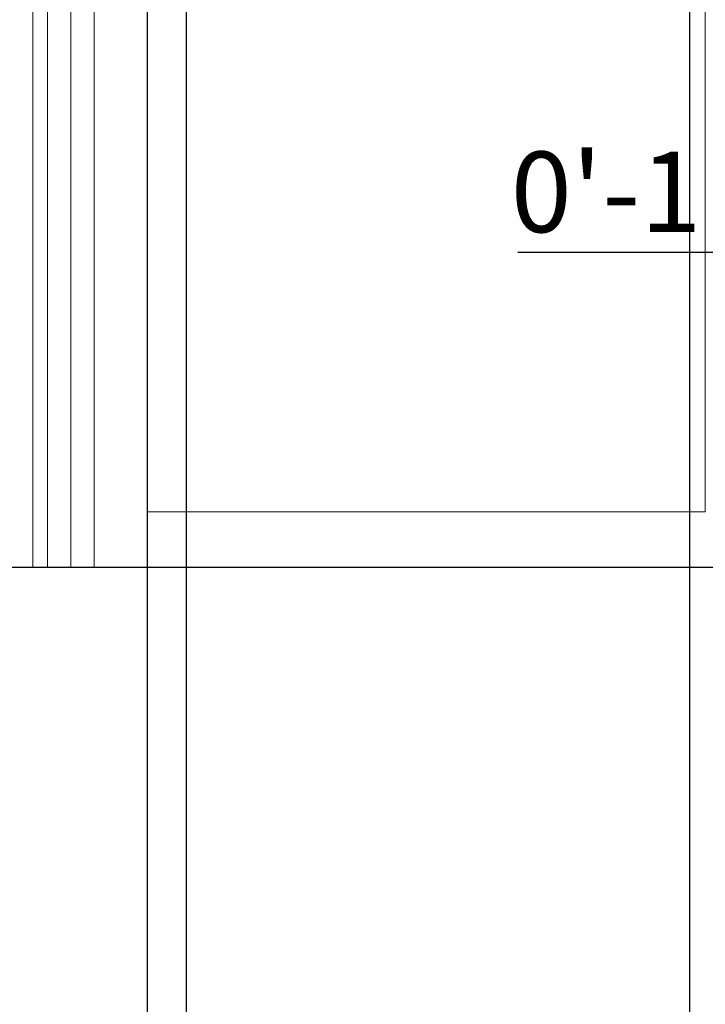
# Model space of a CAD drawing. Units: inches. Extents: x 2656 to 9931, y 1941 to 3068.
# Tile 30 of 46: x 2817 to 2868, y 2855 to 2929. Entities that reach past the tile are written whole.
import ezdxf

# ---------------------------------------------------------------- set-up
doc = ezdxf.new("R2010")
doc.units = ezdxf.units.IN
for name, color, linetype, lineweight in [('A-ANNO-DIMS', 2, 'Continuous', 18), ('A-ELEV', 7, 'Continuous', 25), ('A-ELEV-FNSH', 8, 'Continuous', 13)]:
    doc.layers.add(name, color=color, linetype=linetype, lineweight=lineweight)
doc.styles.get("Standard").update_dxf_attribs({"font": 'arial.ttf'})
doc.dimstyles.new('ISO-25', dxfattribs={"dimtxt": 6, "dimasz": 2.5, "dimexe": 1.25, "dimexo": 0.625, "dimtad": 1, "dimdec": 0, "dimlunit": 3, "dimtxsty": 'Standard', "dimcen": 2.5, "dimadec": 0, "dimazin": 0, "dimtfac": 1, "dimtdec": 0, "dimtmove": 0, "dimatfit": 3, "dimfxl": 1, "dimarcsym": 0})

# ---------------------------------------------------------------- blocks, each defined once
blk = doc.blocks.new('*D63')
at = {"layer": 'A-ANNO-DIMS', "color": 0, "lineweight": -2, "transparency": 16777216}
for p, q in [((2807.088, 2803.318), (2807.088, 2893.004)), ((2799.699, 2803.318), (2808.338, 2803.318)), ((2807.088, 2752.393), (2807.088, 2800.818)), ((2799.699, 2749.893), (2808.338, 2749.893))]:
    blk.add_line(p, q, dxfattribs=at)
at = {"layer": 'A-ANNO-DIMS', "color": 0, "transparency": 16777216}
for points in [[(2806.671, 2800.818), (2807.505, 2800.818), (2807.088, 2803.318)], [(2806.671, 2752.393), (2807.505, 2752.393), (2807.088, 2749.893)]]:
    blk.add_solid(points, dxfattribs=at)
at = {"layer": 'Defpoints', "color": 0, "transparency": 16777216}
for p in [(2799.074, 2803.318), (2807.088, 2803.318), (2799.074, 2749.893)]:
    blk.add_point(p, dxfattribs=at)
at = {"layer": 'A-ANNO-DIMS', "color": 0, "transparency": 16777216, "insert": (2803.358, 2849.411), "char_height": 6, "attachment_point": 5, "rotation": 90}
blk.add_mtext('FRONT GATE 4\'-5 1/2"', dxfattribs=at)
blk = doc.blocks.new('*D151')
at = {"layer": 'A-ANNO-DIMS', "color": 0, "lineweight": -2, "transparency": 16777216}
for p, q in [((2829.546, 2956.424), (2829.546, 2703.709)), ((2867.059, 2955.98), (2867.059, 2703.709)), ((2832.046, 2704.959), (2864.559, 2704.959))]:
    blk.add_line(p, q, dxfattribs=at)
at = {"layer": 'A-ANNO-DIMS', "color": 0, "transparency": 16777216}
for points in [[(2832.046, 2705.376), (2832.046, 2704.543), (2829.546, 2704.959)], [(2864.559, 2705.376), (2864.559, 2704.543), (2867.059, 2704.959)]]:
    blk.add_solid(points, dxfattribs=at)
at = {"layer": 'Defpoints', "color": 0, "transparency": 16777216}
for p in [(2829.546, 2957.049), (2867.059, 2956.605), (2867.059, 2704.959)]:
    blk.add_point(p, dxfattribs=at)
at = {"layer": 'A-ANNO-DIMS', "color": 0, "transparency": 16777216, "insert": (2848.302, 2708.689), "char_height": 6, "attachment_point": 5}
blk.add_mtext('3\'-1 1/2"', dxfattribs=at)
blk = doc.blocks.new('*D153')
at = {"layer": 'A-ANNO-DIMS', "color": 0, "lineweight": -2, "transparency": 16777216}
for p, q in [((2826.64, 2993.722), (2826.64, 2703.709)), ((2829.546, 2956.424), (2829.546, 2703.709)), ((2824.14, 2704.959), (2821.64, 2704.959)), ((2826.64, 2704.959), (2829.546, 2704.959)), ((2832.046, 2704.959), (2851.745, 2704.959))]:
    blk.add_line(p, q, dxfattribs=at)
at = {"layer": 'A-ANNO-DIMS', "color": 0, "transparency": 16777216}
for points in [[(2824.14, 2705.376), (2824.14, 2704.543), (2826.64, 2704.959)], [(2832.046, 2705.376), (2832.046, 2704.543), (2829.546, 2704.959)]]:
    blk.add_solid(points, dxfattribs=at)
at = {"layer": 'Defpoints', "color": 0, "transparency": 16777216}
for p in [(2826.64, 2994.347), (2829.546, 2957.049), (2829.546, 2704.959)]:
    blk.add_point(p, dxfattribs=at)
at = {"layer": 'A-ANNO-DIMS', "color": 0, "transparency": 16777216, "insert": (2843.145, 2708.65), "char_height": 6, "attachment_point": 5}
blk.add_mtext('0\'-3"', dxfattribs=at)
blk = doc.blocks.new('*D163')
at = {"layer": 'A-ANNO-DIMS', "color": 0, "lineweight": -2, "transparency": 16777216}
for p, q in [((2890.428, 2926.692), (2890.428, 2910.117)), ((2891.822, 2926.692), (2891.822, 2910.117)), ((2887.928, 2911.367), (2854.248, 2911.367)), ((2891.822, 2911.367), (2890.428, 2911.367)), ((2894.322, 2911.367), (2896.822, 2911.367))]:
    blk.add_line(p, q, dxfattribs=at)
at = {"layer": 'A-ANNO-DIMS', "color": 0, "transparency": 16777216}
for points in [[(2887.928, 2911.784), (2887.928, 2910.951), (2890.428, 2911.367)], [(2894.322, 2911.784), (2894.322, 2910.951), (2891.822, 2911.367)]]:
    blk.add_solid(points, dxfattribs=at)
at = {"layer": 'Defpoints', "color": 0, "transparency": 16777216}
for p in [(2890.428, 2927.317), (2891.822, 2927.317), (2890.428, 2911.367)]:
    blk.add_point(p, dxfattribs=at)
at = {"layer": 'A-ANNO-DIMS', "color": 0, "transparency": 16777216, "insert": (2869.838, 2915.095), "char_height": 6, "attachment_point": 5}
blk.add_mtext('0\'-1 1/2"', dxfattribs=at)

msp = doc.modelspace()

# ---------------------------------------------------------------- linework, layer by layer
at = {"layer": 'A-ELEV'}
msp.add_line((2998.157, 2887.893), (2743.157, 2887.893), dxfattribs=at)
at = {"layer": 'A-ELEV-FNSH'}
for p, q in [((2818.129, 2887.893), (2818.129, 2998.286)), ((2819.227, 2887.893), (2819.227, 2998.286)), ((2820.954, 2887.893), (2820.954, 2998.286)), ((2822.705, 2887.893), (2822.705, 2998.286))]:
    msp.add_line(p, q, dxfattribs=at)
msp.add_lwpolyline([(2826.64, 2994.347), (2868.226, 2994.347), (2868.226, 2892.035), (2826.64, 2892.035)], close=True, dxfattribs=at)

# ---------------------------------------------------------------- dimensions: what is measured, and where the dimension line sits
at = {"layer": 'A-ANNO-DIMS'}
for base, p1, p2, picture, middle in [((2829.546, 2704.959), (2826.64, 2994.347), (2829.546, 2957.049), '*D153', (2843.145, 2708.65)), ((2867.059, 2704.959), (2829.546, 2957.049), (2867.059, 2956.605), '*D151', (2848.302, 2708.689))]:
    dim = msp.add_linear_dim(base=base, p1=p1, p2=p2, dimstyle='ISO-25', override={"dimdec": 1, "dimlfac": 1, "dimrnd": 0, "dimzin": 1, "dimdsep": 46, "dimlunit": 4, "dimfrac": 2}, dxfattribs=at)
    dim.commit()
    dim.dimension.update_dxf_attribs({"geometry": picture, "text_midpoint": middle})
dim = msp.add_linear_dim(base=(2890.428, 2911.367), p1=(2891.822, 2927.317), p2=(2890.428, 2927.317), angle=180, dimstyle='ISO-25', override={"dimdec": 1, "dimlfac": 1, "dimrnd": 0, "dimzin": 1, "dimdsep": 46, "dimlunit": 4, "dimfrac": 2}, dxfattribs=at)
dim.commit()
dim.dimension.update_dxf_attribs({"geometry": '*D163', "text_midpoint": (2869.838, 2915.095)})
dim = msp.add_linear_dim(base=(2807.088, 2803.318), p1=(2799.074, 2749.893), p2=(2799.074, 2803.318), angle=90, text='FRONT GATE <>', dimstyle='ISO-25', override={"dimdec": 1, "dimlfac": 1, "dimrnd": 0, "dimzin": 1, "dimdsep": 46, "dimlunit": 4, "dimfrac": 2}, dxfattribs=at)
dim.commit()
dim.dimension.update_dxf_attribs({"geometry": '*D63', "text_midpoint": (2803.358, 2849.411)})

doc.saveas('drawing.dxf')
